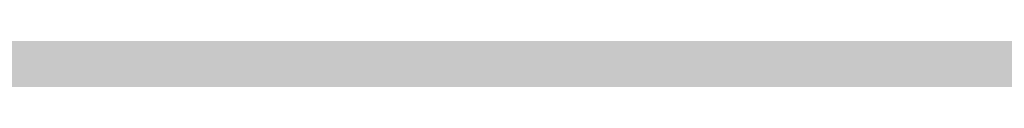
# Model space of a CAD drawing. Units: inches. Extents: x 2083 to 3317, y 1141 to 2115.
# Tile 152 of 256: x 3126.946713 to 3126.955939, y 1263.261646 to 1263.261932. Entities that reach past the tile are written whole.
import ezdxf

# ---------------------------------------------------------------- set-up
doc = ezdxf.new("R2010")
doc.units = ezdxf.units.IN
doc.layers.add('A-ANNO-DIMS', color=2, linetype='Continuous', lineweight=18)
doc.layers.add('A-WALL-PATT', color=251, linetype='Continuous', lineweight=13, true_color=0x636466)
doc.styles.get("Standard").update_dxf_attribs({"font": 'arial.ttf'})
doc.dimstyles.new('ISO-25', dxfattribs={"dimtxt": 12, "dimasz": 12, "dimexe": 1.25, "dimexo": 0.625, "dimtad": 1, "dimlunit": 3, "dimtxsty": 'Standard', "dimcen": 2.5, "dimadec": 0, "dimazin": 0, "dimtfac": 1, "dimtmove": 0, "dimatfit": 3, "dimfxl": 1, "dimarcsym": 0})

# ---------------------------------------------------------------- blocks, each defined once
blk = doc.blocks.new('*D26')
at = {"layer": 'A-ANNO-DIMS', "color": 0, "lineweight": -2, "transparency": 16777216}
for p, q in [((3088.985844, 1274.915092), (3088.985844, 1270.9519631)), ((3111.2400366, 1274.915092), (3111.2400366, 1270.9519631)), ((3076.985844, 1272.2019631), (2840.262447, 1272.2019631)), ((3111.2400366, 1272.2019631), (3088.985844, 1272.2019631)), ((3123.2400366, 1272.2019631), (3135.2400366, 1272.2019631))]:
    blk.add_line(p, q, dxfattribs=at)
at = {"layer": 'A-ANNO-DIMS', "color": 0, "transparency": 16777216}
for points in [[(3076.985844, 1274.2019631), (3076.985844, 1270.2019631), (3088.985844, 1272.2019631)], [(3123.2400366, 1274.2019631), (3123.2400366, 1270.2019631), (3111.2400366, 1272.2019631)]]:
    blk.add_solid(points, dxfattribs=at)
at = {"layer": 'Defpoints', "color": 0, "transparency": 16777216}
for p in [(3088.985844, 1275.540092), (3111.2400366, 1275.540092), (3088.985844, 1272.2019631)]:
    blk.add_point(p, dxfattribs=at)
at = {"layer": 'A-ANNO-DIMS', "color": 0, "transparency": 16777216, "insert": (2952.6241455, 1279.0316016), "char_height": 12, "attachment_point": 5}
blk.add_mtext('NIGHTSTAND 1\'-10 1/2" TYP.', dxfattribs=at)

msp = doc.modelspace()

# ---------------------------------------------------------------- hatches: boundary and pattern name
at = {"layer": 'A-WALL-PATT'}
h = msp.add_hatch(color=256, dxfattribs=at)
h.dxf.hatch_style = 1
h.paths.add_polyline_path([(3126.9597832, 2020.7613601), (2748.9597832, 2020.7613601), (2604.9597832, 2020.7613601), (2226.9597832, 2020.7613601), (2226.9597832, 1702.7613601), (2466.9597832, 1702.7613601), (2466.9597832, 1582.7613601), (2418.9597832, 1582.7613601), (2418.9597832, 1477.7613601), (2226.9597832, 1477.7613601), (2226.9597832, 1263.2613601), (2544.9597832, 1263.2613601), (2544.9597832, 1411.7613601), (2604.9597832, 1411.7613601), (2685.9597832, 1411.7613601), (2685.9597832, 1420.7613601), (2604.9597832, 1420.7613601), (2604.9597832, 1573.7613601), (2604.9597832, 1702.7613601), (2604.9597832, 2011.7613601), (2748.9597832, 2011.7613601), (2748.9597832, 1702.7613601), (2862.9597832, 1702.7613601), (2862.9597832, 1621.7613601), (2871.9597832, 1621.7613601), (2871.9597832, 1702.7613601), (2883.9597832, 1702.7613601), (2883.9597832, 1706.9394595, -0.026459), (2883.9597832, 1711.7613601), (2757.9597832, 1711.7613601), (2757.9597832, 1807.7613601), (2787.9597832, 1807.7613601), (2787.9597832, 1812.2613601), (2757.9597832, 1812.2613601), (2757.9597832, 2011.7613601), (2877.9597832, 2011.7613601), (2877.9597832, 1812.2613601), (2847.9597832, 1812.2613601), (2847.9597832, 1807.7613601), (2889.8357425, 1807.7613601), (2889.8357425, 1812.2613601), (2882.4597832, 1812.2613601), (2882.4597832, 2011.7613601), (3117.9597832, 2011.7613601), (3117.9597832, 1812.2613601), (2937.8357425, 1812.2613601), (2937.8357425, 1807.7613601), (2995.7097832, 1807.7613601), (2995.7097832, 1796.1176655), (3000.2097832, 1796.1176655), (3000.2097832, 1807.7613601), (3117.9597832, 1807.7613601), (3117.9597832, 1711.7613601), (3000.2097832, 1711.7613601), (3000.2097832, 1760.1176655), (2998.5727047, 1760.1176655, -0.020711), (2995.7097832, 1760.1176655), (2995.7097832, 1711.7613601), (2931.9597832, 1711.7613601), (2931.9597832, 1702.7613601), (3126.9597832, 1702.7613601)])
h.paths.add_polyline_path([(2471.4597832, 2011.7613601), (2471.4597832, 1810.0113601), (2462.7169357, 1810.0113601), (2462.7169357, 1805.5113601), (2505.9597832, 1805.5113601), (2505.9597832, 1810.0113601), (2475.9597832, 1810.0113601), (2475.9597832, 2011.7613601), (2595.9597832, 2011.7613601), (2595.9597832, 1810.0113601), (2565.9597832, 1810.0113601), (2565.9597832, 1805.5113601), (2595.9597832, 1805.5113601), (2595.9597832, 1711.7613601), (2235.9597832, 1711.7613601), (2235.9597832, 1805.5113601), (2353.7097832, 1805.5113601), (2353.7097832, 1796.0541624), (2358.2097832, 1796.0541624), (2358.2097832, 1805.5113601), (2414.7169357, 1805.5113601), (2414.7169357, 1810.0113601), (2235.9597832, 1810.0113601), (2235.9597832, 2011.7613601)], flags=16)
h.paths.add_polyline_path([(2270.2047343, 1994.6100082), (2270.2047343, 1970.6100082), (2246.2047343, 1970.6100082), (2246.2047343, 1994.6100082)], flags=0)
edge = h.paths.add_edge_path(flags=0)
edge.add_ellipse((2332.027391, 1899.7981761), major_axis=(-3.0429938, 3.0429938), ratio=0.16825245, start_angle=-161.3321656, end_angle=-156.3071136, ccw=False)
edge.add_ellipse((2333.0820373, 1898.7435297), major_axis=(-1.0546463, 1.0546463), ratio=0.453532097, start_angle=-123.371019, end_angle=-94.1591066)
edge = h.paths.add_edge_path(flags=0)
edge.add_ellipse((2332.027391, 1968.8762897), major_axis=(3.0429938, 3.0429938), ratio=0.16825245, start_angle=18.6678344, end_angle=23.6928864)
edge.add_spline(control_points=[(2332.9255964, 1970.6911045), (2332.2267681, 1970.3360997), (2330.8937087, 1969.6589054), (2328.4130803, 1970.9321376), (2327.2039345, 1967.7487119), (2324.7095965, 1969.9555886), (2322.5328223, 1967.012354), (2320.0128462, 1971.2958124), (2317.6803077, 1968.1578449), (2316.0405263, 1967.1020468), (2315.4269045, 1966.8096022)], knot_values=[0, 0, 0, 0, 2.267059, 4.324559, 6.685584, 8.878641, 11.121502, 14.300359, 17.755284, 19.732645, 19.732645, 19.732645, 19.732645], degree=3, periodic=0)
edge.add_ellipse((2332.027391, 1968.8762897), major_axis=(3.0429938, 3.0429938), ratio=0.16825245, start_angle=18.6678344, end_angle=23.6928864, ccw=False)
edge.add_ellipse((2333.0820373, 1969.930936), major_axis=(1.0546463, 1.0546463), ratio=0.453532097, start_angle=56.628981, end_angle=85.8408934, ccw=False)
edge = h.paths.add_edge_path(flags=0)
edge.add_spline(control_points=[(2296.4282874, 1967.9879081), (2293.6278045, 1965.3363137), (2287.7036238, 1959.727094), (2299.7438601, 1949.9956993), (2294.5325909, 1935.6685275), (2290.5732281, 1920.6035119), (2293.3941244, 1909.9736911), (2296.1854073, 1904.9665431)], knot_values=[0.099185, 0.099185, 0.099185, 0.099185, 0.345301, 0.619822, 0.982653, 1.386093, 1.810555, 1.810555, 1.810555, 1.810555], degree=3, periodic=0)
edge.add_spline(control_points=[(2296.1854073, 1904.9665431), (2297.3835817, 1902.6193002), (2298.0009694, 1901.9493116), (2298.5529698, 1901.4681549)], knot_values=[0.006246, 0.006246, 0.006246, 0.006246, 0.055476, 0.055476, 0.055476, 0.055476], degree=3, periodic=0)
edge.add_spline(control_points=[(2298.5529698, 1901.4681549), (2297.2586121, 1900.9232238), (2295.2252939, 1900.2321257), (2293.0602287, 1900.6142053), (2292.1014227, 1900.788415), (2292.0895776, 1900.790568)], knot_values=[0.312835, 0.312835, 0.312835, 0.312835, 0.40178, 0.474987, 0.475903, 0.475903, 0.475903, 0.475903], degree=3, periodic=0)
edge.add_arc((2292.7936464, 1904.6641088), 3.9370079, 215.4208969, 259.6981795, ccw=False)
edge.add_spline(control_points=[(2289.5853139, 1902.3823039), (2289.4766524, 1902.5350874), (2289.3684805, 1902.6880353), (2289.2608648, 1902.8411699)], knot_values=[0.102872, 0.102872, 0.102872, 0.102872, 0.116896, 0.116896, 0.116896, 0.116896], degree=3, periodic=0)
edge.add_spline(control_points=[(2289.2608648, 1902.8411699), (2288.6866042, 1902.5501922), (2287.6400477, 1902.0199025), (2285.8813368, 1901.8739536), (2283.8529717, 1901.5043521), (2281.7199871, 1899.7105375), (2278.4669913, 1899.492942), (2276.1571361, 1901.8832022), (2272.2589526, 1899.8040711), (2267.7776054, 1901.8431828), (2262.2438819, 1900.1840326), (2257.414927, 1901.7820606), (2254.318374, 1900.7261196), (2253.1782849, 1900.3373431)], knot_values=[0, 0, 0, 0, 1.907977, 3.477176, 5.261074, 7.972851, 11.680248, 13.717921, 16.939592, 22.789562, 27.502503, 33.595215, 37.145618, 37.145618, 37.145618, 37.145618], degree=3, periodic=0)
edge.add_line((2253.1782849, 1900.3373431), (2250.2442397, 1902.8411699))
edge.add_line((2250.2442397, 1902.8411699), (2250.2442397, 1965.8332959))
edge.add_line((2250.2442397, 1965.8332959), (2253.1782849, 1968.3371226))
edge.add_spline(control_points=[(2253.1782849, 1968.3371226), (2254.318374, 1967.9483462), (2257.414927, 1966.8924051), (2262.2438819, 1968.4904332), (2267.7776054, 1966.8312829), (2271.5267301, 1968.5372172), (2273.8759143, 1967.8282895), (2274.2067012, 1967.7276424)], knot_values=[0, 0, 0, 0, 0.09018, 0.244935, 0.364644, 0.513233, 0.537855, 0.537855, 0.537855, 0.537855], degree=3, periodic=0)
edge.add_arc((2274.3528869, 1963.7933495), 3.9370079, 72.0511336, 92.1279492, ccw=False)
edge.add_arc((2281.2969331, 1985.2300027), 18.5962982, 252.05113361, 288.56572166)
edge.add_arc((2292.3167172, 1956.0288805), 12.6460805, 71.02678788, 113.77821843, ccw=False)
edge = h.paths.add_edge_path(flags=0)
edge.add_spline(control_points=[(2274.8994147, 1951.8561946), (2275.066156, 1951.6165924), (2275.2326866, 1951.3765878), (2275.3979871, 1951.1358545)], knot_values=[1.409916, 1.409916, 1.409916, 1.409916, 1.43159, 1.43159, 1.43159, 1.43159], degree=3, periodic=0)
edge.add_spline(control_points=[(2275.3979871, 1951.1358545), (2275.7921055, 1950.5618854), (2276.1792311, 1949.9837745), (2276.5455462, 1949.3971029)], knot_values=[1.358238, 1.358238, 1.358238, 1.358238, 1.409916, 1.409916, 1.409916, 1.409916], degree=3, periodic=0)
edge.add_line((2276.5455462, 1949.3971029), (2277.437289, 1947.8621847))
edge.add_spline(control_points=[(2277.437289, 1947.8621847), (2276.3038341, 1945.6731147), (2274.6396979, 1942.4268817), (2274.631615, 1938.0938998), (2272.7991237, 1930.8515498), (2274.3564261, 1943.8970461), (2275.9476814, 1947.9233558), (2276.5455462, 1949.3971029)], knot_values=[0.005632, 0.005632, 0.005632, 0.005632, 0.186014, 0.266002, 0.357087, 0.59639, 0.739732, 0.739732, 0.739732, 0.739732], degree=3, periodic=0)
edge.add_spline(control_points=[(2276.5455462, 1949.3971029), (2276.1792311, 1949.9837745), (2275.7921055, 1950.5618854), (2275.3979871, 1951.1358545)], knot_values=[1.358238, 1.358238, 1.358238, 1.358238, 1.409916, 1.409916, 1.409916, 1.409916], degree=3, periodic=0)
edge.add_spline(control_points=[(2275.3979871, 1951.1358545), (2274.9425002, 1950.0804523), (2274.2077604, 1948.0252718), (2273.9346018, 1944.8514774), (2272.4685341, 1937.6274891), (2273.4662155, 1945.6964663), (2274.7006154, 1951.0594725), (2274.8994147, 1951.8561946)], knot_values=[0.104364, 0.104364, 0.104364, 0.104364, 0.189636, 0.269624, 0.36071, 0.600013, 0.644622, 0.644622, 0.644622, 0.644622], degree=3, periodic=0)
h.paths.add_polyline_path([(2269.1675139, 1963.1275729, -0.357527), (2268.170633, 1960.9763695, -0.092561), (2268.170633, 1939.4363249, -0.357527), (2269.1675139, 1937.2851215, -0.357527), (2267.0163105, 1938.2820024, -0.164785), (2254.6855813, 1938.2820024, -0.357527), (2252.5343779, 1937.2851215, -0.357527), (2253.5312587, 1939.4363249, -0.092561), (2253.5312587, 1960.9763695, -0.357527), (2252.5343779, 1963.1275729, -0.357527), (2254.6855813, 1962.130692, -0.164785), (2267.0163105, 1962.130692, -0.357527)], flags=0)
h.paths.add_polyline_path([(2248.8740679, 1967.8017998), (2248.8740679, 1957.0277095), (2249.4577833, 1957.0277095), (2249.4577833, 1911.6467562), (2248.8740679, 1911.6467562), (2248.8740679, 1900.8726659), (2246.5118632, 1900.8726659, 0.197327), (2244.1496584, 1902.4568734), (2244.1496584, 1966.2175923, 0.197327), (2246.5118632, 1967.8017998)], flags=0)
h.paths.add_polyline_path([(2269.1675139, 1931.3893442, -0.357527), (2268.170633, 1929.2381408, -0.092561), (2268.170633, 1907.6980962, -0.357527), (2269.1675139, 1905.5468928, -0.357527), (2267.0163105, 1906.5437737, -0.164785), (2254.6855813, 1906.5437737, -0.357527), (2252.5343779, 1905.5468928, -0.357527), (2253.5312587, 1907.6980962, -0.092561), (2253.5312587, 1929.2381408, -0.357527), (2252.5343779, 1931.3893442, -0.357527), (2254.6855813, 1930.3924634, -0.164785), (2267.0163105, 1930.3924634, -0.357527)], flags=0)
edge = h.paths.add_edge_path(flags=0)
edge.add_spline(control_points=[(2276.1968578, 1906.7237016), (2276.1681442, 1909.0289278), (2276.1140492, 1913.371852), (2270.5984171, 1924.9249783), (2273.9051746, 1919.0127787), (2275.9217115, 1916.2620626), (2275.4745699, 1912.4021495), (2277.2578735, 1910.3806206), (2276.6960436, 1908.2250358), (2276.6462176, 1906.8130226), (2276.6178249, 1906.0084068)], knot_values=[0, 0, 0, 0, 8.61026, 16.221274, 18.843057, 23.804898, 27.440828, 29.356102, 31.203478, 33.650687, 33.650687, 33.650687, 33.650687], degree=3, periodic=0)
edge.add_spline(control_points=[(2276.6178249, 1906.0084068), (2276.6233131, 1905.6241436), (2276.4977381, 1904.6286608), (2275.4417789, 1903.8547251), (2274.9373144, 1903.0804497), (2274.8590804, 1902.8411699)], knot_values=[0.156488, 0.156488, 0.156488, 0.156488, 0.184398, 0.231376, 0.250598, 0.250598, 0.250598, 0.250598], degree=3, periodic=0)
edge.add_line((2274.8590804, 1902.8411699), (2276.50598, 1902.8411699))
edge.add_spline(control_points=[(2276.50598, 1902.8411699), (2276.7883084, 1903.0849395), (2277.6650711, 1904.1251958), (2278.2495378, 1904.340738), (2277.6538719, 1908.5273866), (2278.15567, 1906.2278078), (2278.100464, 1905.2859484), (2278.8466748, 1904.0690054), (2277.8567853, 1903.4149482), (2277.8741909, 1902.9910497), (2277.9035616, 1902.8411699)], knot_values=[0.059574, 0.059574, 0.059574, 0.059574, 0.080753, 0.103741, 0.16972, 0.176036, 0.207137, 0.240474, 0.262341, 0.27366, 0.27366, 0.27366, 0.27366], degree=3, periodic=0)
edge.add_line((2277.9035616, 1902.8411699), (2280.0298255, 1902.8411699))
edge.add_spline(control_points=[(2280.0298255, 1902.8411699), (2279.8882214, 1903.088398), (2279.4992571, 1903.9815512), (2280.1522839, 1905.9393491), (2278.103615, 1909.6577572), (2279.7623946, 1907.185285), (2280.3279002, 1904.8748608), (2280.4851086, 1903.4895904), (2281.4632687, 1903.2494323), (2281.7583431, 1902.9364967), (2281.8340361, 1902.8411699)], knot_values=[0.013856, 0.013856, 0.013856, 0.013856, 0.034874, 0.088867, 0.107879, 0.126738, 0.158714, 0.193757, 0.217487, 0.226722, 0.226722, 0.226722, 0.226722], degree=3, periodic=0)
edge.add_spline(control_points=[(2281.8340361, 1902.8411699), (2281.7875348, 1902.8267029), (2281.6470224, 1902.7829881), (2281.3955272, 1902.85949), (2281.088077, 1902.9852418), (2280.7206826, 1903.060902), (2280.3334513, 1903.0257257), (2280.1247668, 1902.898879), (2280.0298255, 1902.8411699)], knot_values=[0, 0, 0, 0, 0.14413, 0.435517, 0.749276, 1.153046, 1.548371, 1.878348, 1.878348, 1.878348, 1.878348], degree=3, periodic=0)
edge.add_line((2280.0298255, 1902.8411699), (2277.9035616, 1902.8411699))
edge.add_spline(control_points=[(2277.9035616, 1902.8411699), (2277.892855, 1902.7958553), (2277.865396, 1902.6796374), (2277.6074793, 1902.6874828), (2277.2740503, 1902.8006999), (2276.8379209, 1902.6197745), (2276.5838074, 1902.7892611), (2276.50598, 1902.8411699)], knot_values=[0, 0, 0, 0, 0.127189, 0.326199, 0.628009, 1.24357, 1.515331, 1.515331, 1.515331, 1.515331], degree=3, periodic=0)
edge.add_line((2276.50598, 1902.8411699), (2274.8590804, 1902.8411699))
edge.add_spline(control_points=[(2274.8590804, 1902.8411699), (2274.8144367, 1902.8985868), (2274.7251297, 1903.013446), (2274.4934765, 1903.1189684), (2274.2442854, 1902.9605386), (2273.9371207, 1903.1849416), (2273.6140395, 1902.9831428), (2273.4083164, 1902.8830449), (2273.322254, 1902.8411699)], knot_values=[0, 0, 0, 0, 0.21843, 0.436957, 0.687977, 0.990379, 1.398396, 1.69185, 1.69185, 1.69185, 1.69185], degree=3, periodic=0)
edge.add_spline(control_points=[(2273.322254, 1902.8411699), (2273.6167403, 1903.445692), (2274.2739977, 1904.5382529), (2276.0272387, 1904.5737017), (2276.2069634, 1906.5836372), (2276.1968578, 1906.7237016)], knot_values=[0.012227, 0.012227, 0.012227, 0.012227, 0.059472, 0.106218, 0.134458, 0.134458, 0.134458, 0.134458], degree=3, periodic=0)
h.paths.add_polyline_path([(2270.7760538, 1897.7898284), (2270.7760538, 1873.7898284), (2246.7760538, 1873.7898284), (2246.7760538, 1897.7898284)], flags=0)
h.paths.add_polyline_path([(2353.7097832, 1760.0050593), (2353.7097832, 1760.0541624), (2358.2097832, 1760.0541624, -0.033729)], flags=0)
h.paths.add_polyline_path([(2321.8191188, 1737.5291862), (2341.9953271, 1737.5291862, -0.414214), (2343.2032727, 1736.3212406), (2343.2032727, 1721.0205964, -0.414214), (2341.9953271, 1719.8126508), (2321.8191188, 1719.8126508, -0.414214), (2320.6111732, 1721.0205964), (2320.6111732, 1736.3212406, -0.414214)], flags=0)
h.paths.add_polyline_path([(2324.2350099, 1736.3212406), (2339.5794359, 1736.3212406, -0.414214), (2341.9953271, 1733.9053494), (2341.9953271, 1725.4497302, -0.414214), (2339.5794359, 1723.033839), (2333.6805885, 1723.033839), (2333.8453172, 1722.0454666, -0.870646), (2335.4253988, 1721.8258934, -0.767327), (2333.922694, 1721.4232449), (2331.2910241, 1721.4232449, -0.767327), (2329.7883193, 1721.8258934, -0.870646), (2331.3684009, 1722.0454666), (2331.5331296, 1723.033839), (2324.2350099, 1723.033839, -0.414214), (2321.8191188, 1725.4497302), (2321.8191188, 1733.9053494, -0.414214)], flags=0)
h.paths.add_polyline_path([(2570.4837892, 1928.6154443), (2589.6837892, 1928.6154443), (2590.1688286, 1928.6154443), (2590.1688286, 1904.9933971), (2570.4837892, 1904.9933971)], flags=0)
h.paths.add_polyline_path([(2574.4473242, 1927.2638215, -1), (2572.8288357, 1927.2638215, -1)], flags=0)
h.paths.add_polyline_path([(2573.0898665, 1926.9408768), (2573.925032, 1927.7760423), (2574.1477428, 1927.5533315), (2573.3125773, 1926.718166)], flags=0)
h.paths.add_polyline_path([(2578.7790648, 1919.7296175, -1), (2571.5916632, 1919.7296175, -1)], flags=0)
h.paths.add_polyline_path([(2578.385364, 1919.7296175, -1), (2571.985364, 1919.7296175, -1)], flags=0)
h.paths.add_polyline_path([(2331.5957638, 1729.4762156, -1), (2333.6179542, 1729.4762156, -1)], flags=0)
h.paths.add_polyline_path([(2578.0342282, 1927.2638215, -1), (2576.4157396, 1927.2638215, -1)], flags=0)
h.paths.add_polyline_path([(2576.6888513, 1927.5310886), (2576.9115621, 1927.7537993), (2577.7467276, 1926.9186339), (2577.5240168, 1926.6959231)], flags=0)
h.paths.add_polyline_path([(2578.1390648, 1909.8595388, -1), (2572.2316632, 1909.8595388, -1)], flags=0)
h.paths.add_polyline_path([(2577.745364, 1909.8595388, -1), (2572.625364, 1909.8595388, -1)], flags=0)
h.paths.add_polyline_path([(2583.7977179, 1927.2638215, -1), (2582.1792294, 1927.2638215, -1)], flags=0)
h.paths.add_polyline_path([(2582.7186487, 1927.7537993), (2583.5538142, 1926.9186339), (2583.3311034, 1926.6959231), (2582.4959379, 1927.5310886)], flags=0)
h.paths.add_polyline_path([(2582.4959379, 1927.5310886), (2582.7186487, 1927.7537993), (2583.5538142, 1926.9186339), (2583.3311034, 1926.6959231)], flags=0)
h.paths.add_polyline_path([(2587.7390648, 1920.5296175, -1), (2581.8316632, 1920.5296175, -1)], flags=0)
h.paths.add_polyline_path([(2587.345364, 1920.5296175, -1), (2582.225364, 1920.5296175, -1)], flags=0)
h.paths.add_polyline_path([(2587.3846219, 1927.2638215, -1), (2585.7661333, 1927.2638215, -1)], flags=0)
h.paths.add_polyline_path([(2586.0819925, 1926.9802469), (2586.917158, 1927.8154124), (2587.1398688, 1927.5927016), (2586.3047033, 1926.7575361)], flags=0)
h.paths.add_polyline_path([(2588.3790648, 1910.6595388, -1), (2581.1916632, 1910.6595388, -1)], flags=0)
h.paths.add_polyline_path([(2587.985364, 1910.6595388, -1), (2581.585364, 1910.6595388, -1)], flags=0)
h.paths.add_polyline_path([(2417.1677288, 1729.4778955), (2437.3439372, 1729.4778955, -0.414214), (2438.5518828, 1728.2699499), (2438.5518828, 1712.9693057, -0.414214), (2437.3439372, 1711.7613601), (2417.1677288, 1711.7613601, -0.414214), (2415.9597832, 1712.9693057), (2415.9597832, 1728.2699499, -0.414214)], flags=0)
h.paths.add_polyline_path([(2419.58362, 1728.2699499), (2434.928046, 1728.2699499, -0.414214), (2437.3439372, 1725.8540587), (2437.3439372, 1717.3984395, -0.414214), (2434.928046, 1714.9825483), (2429.0291985, 1714.9825483), (2429.1939273, 1713.9941758, -0.870646), (2430.7740089, 1713.7746027, -0.767327), (2429.2713041, 1713.3719542), (2426.6396342, 1713.3719542, -0.767327), (2425.1369294, 1713.7746027, -0.870646), (2426.717011, 1713.9941758), (2426.8817397, 1714.9825483), (2419.58362, 1714.9825483, -0.414214), (2417.1677288, 1717.3984395), (2417.1677288, 1725.8540587, -0.414214)], flags=0)
h.paths.add_polyline_path([(2419.58362, 1728.2699499), (2434.928046, 1728.2699499, -0.414214), (2437.3439372, 1725.8540587), (2437.3439372, 1717.3984395, -0.414214), (2434.928046, 1714.9825483), (2429.0291985, 1714.9825483), (2428.3581177, 1719.0090337), (2427.5528206, 1719.0090337), (2426.8817397, 1714.9825483), (2419.58362, 1714.9825483, -0.414214), (2417.1677288, 1717.3984395), (2417.1677288, 1725.8540587, -0.414214)], flags=0)
h.paths.add_polyline_path([(2426.9443739, 1721.4249248, -1), (2428.9665643, 1721.4249248, -1)], flags=0)
h.paths.add_polyline_path([(2475.9597832, 1702.7613601), (2595.9597832, 1702.7613601), (2595.9597832, 1582.7613601), (2475.9597832, 1582.7613601)], flags=16)
h.paths.add_polyline_path([(2427.9597832, 1573.7613601), (2595.9597832, 1573.7613601), (2595.9597832, 1468.7613601), (2595.9597832, 1420.7613601), (2384.4597832, 1420.7613601), (2384.4597832, 1468.7613601), (2427.9597832, 1468.7613601)], flags=16)
h.paths.add_polyline_path([(2379.9597832, 1468.7613601), (2379.9597832, 1420.7613601), (2235.9597832, 1420.7613601), (2235.9597832, 1468.7613601)], flags=16)
h.paths.add_polyline_path([(2317.8159962, 1466.695767), (2337.9922045, 1466.695767, -0.414214), (2339.2001501, 1465.4878214), (2339.2001501, 1450.1871771, -0.414214), (2337.9922045, 1448.9792315), (2317.8159962, 1448.9792315, -0.414214), (2316.6080506, 1450.1871771), (2316.6080506, 1465.4878214, -0.414214)], flags=0)
h.paths.add_polyline_path([(2320.2318874, 1465.4878214), (2335.5763133, 1465.4878214, -0.414214), (2337.9922045, 1463.0719302), (2337.9922045, 1454.616311, -0.414214), (2335.5763133, 1452.2004198), (2329.6774659, 1452.2004198), (2329.8421946, 1451.2120473, -0.870646), (2331.4222762, 1450.9924742, -0.767327), (2329.9195714, 1450.5898257), (2327.2879015, 1450.5898257, -0.767327), (2325.7851967, 1450.9924742, -0.870646), (2327.3652783, 1451.2120473), (2327.530007, 1452.2004198), (2320.2318874, 1452.2004198, -0.414214), (2317.8159962, 1454.616311), (2317.8159962, 1463.0719302, -0.414214)], flags=0)
h.paths.add_polyline_path([(2320.2318874, 1465.4878214), (2335.5763133, 1465.4878214, -0.414214), (2337.9922045, 1463.0719302), (2337.9922045, 1454.616311, -0.414214), (2335.5763133, 1452.2004198), (2329.6774659, 1452.2004198), (2329.006385, 1456.2269051), (2328.2010879, 1456.2269051), (2327.530007, 1452.2004198), (2320.2318874, 1452.2004198, -0.414214), (2317.8159962, 1454.616311), (2317.8159962, 1463.0719302, -0.414214)], flags=0)
h.paths.add_polyline_path([(2327.5926413, 1458.6427963, -1), (2329.6148317, 1458.6427963, -1)], flags=0)
h.paths.add_polyline_path([(2244.4117436, 1433.3404531), (2241.9209449, 1433.3404531, -0.414214), (2240.0178562, 1435.2435418), (2240.0178562, 1440.9528078, -0.414211), (2241.920925, 1442.8558965), (2244.4117436, 1442.8558965, -1.976472)], flags=0)
h.paths.add_polyline_path([(2245.3568884, 1434.3975358, -0.414214), (2245.3568884, 1441.7988138, -2.144098)], flags=0)
h.paths.add_polyline_path([(2535.9597832, 1416.2613601), (2535.9597832, 1272.2613601), (2235.9597832, 1272.2613601), (2235.9597832, 1416.2613601)], flags=16)
h.paths.add_polyline_path([(2260.1195614, 1384.2928413), (2260.1195614, 1362.0386487), (2237.8653688, 1362.0386487), (2237.8653688, 1384.2928413)], flags=0)
edge = h.paths.add_edge_path(flags=0)
edge.add_line((2318.2518466, 1362.0932983), (2318.1457968, 1362.0009726))
edge.add_ellipse((2317.4451158, 1360.4310442), major_axis=(2.8216404, 2.8216404), ratio=0.16825245, start_angle=18.6678344, end_angle=20.9481273, ccw=False)
edge.add_ellipse((2318.4230451, 1361.4089735), major_axis=(0.9779293, 0.9779293), ratio=0.453532097, start_angle=56.628981, end_angle=70.2262012, ccw=False)
edge = h.paths.add_edge_path(flags=0)
edge.add_line((2319.1073699, 1295.5710784), (2319.0150442, 1295.6771282))
edge.add_ellipse((2317.4451158, 1296.3778091), major_axis=(-2.8216404, 2.8216404), ratio=0.16825245, start_angle=-161.3321656, end_angle=-159.0518727, ccw=False)
edge.add_ellipse((2318.4230451, 1295.3998798), major_axis=(-0.9779293, 0.9779293), ratio=0.453532097, start_angle=-123.371019, end_angle=-109.7737988)
edge = h.paths.add_edge_path(flags=0)
edge.add_spline(control_points=[(2284.2103489, 1301.1702189), (2284.5806878, 1300.444719), (2284.8911891, 1299.8920243), (2285.159553, 1299.4610182)], knot_values=[0.039066, 0.039066, 0.039066, 0.039066, 0.055476, 0.055476, 0.055476, 0.055476], degree=3, periodic=0)
edge.add_line((2285.159553, 1299.4610182), (2284.2103489, 1301.1702189))
edge = h.paths.add_edge_path(flags=0)
edge.add_line((2280.4124579, 1297.2980125), (2283.3699905, 1297.0361216))
edge.add_line((2283.3699905, 1297.0361216), (2286.4056902, 1297.9263104))
edge.add_spline(control_points=[(2286.4056902, 1297.9263104), (2285.305487, 1297.4631193), (2284.3447774, 1297.1291508), (2283.3699905, 1297.0361216)], knot_values=[0.394369, 0.394369, 0.394369, 0.394369, 0.475903, 0.475903, 0.475903, 0.475903], degree=3, periodic=0)
edge.add_spline(control_points=[(2283.3699905, 1297.0361216), (2283.2813895, 1297.027666), (2282.316289, 1296.9573356), (2281.3125019, 1297.1344787), (2280.4234414, 1297.2960161), (2280.4124579, 1297.2980125)], knot_values=[0.312835, 0.312835, 0.312835, 0.312835, 0.320246, 0.393453, 0.394369, 0.394369, 0.394369, 0.394369], degree=3, periodic=0)
edge = h.paths.add_edge_path(flags=0)
edge.add_line((2284.4355615, 1359.6072854), (2280.4462909, 1355.328047))
edge.add_line((2280.4462909, 1355.328047), (2279.5799868, 1351.0177544))
edge.add_line((2279.5799868, 1351.0177544), (2282.4129737, 1346.5804327))
edge.add_spline(control_points=[(2282.4129737, 1346.5804327), (2283.1533308, 1345.5892358), (2284.2528957, 1344.0288973), (2284.801037, 1342.3871671), (2284.9351625, 1341.8055443)], knot_values=[1.240098, 1.240098, 1.240098, 1.240098, 1.332892, 1.382712, 1.382712, 1.382712, 1.382712], degree=3, periodic=0)
edge.add_spline(control_points=[(2284.9351625, 1341.8055443), (2285.3191079, 1340.1406002), (2285.2330291, 1338.4092041), (2284.9099384, 1336.6541222)], knot_values=[1.097484, 1.097484, 1.097484, 1.097484, 1.240098, 1.240098, 1.240098, 1.240098], degree=3, periodic=0)
edge.add_spline(control_points=[(2284.9099384, 1336.6541222), (2284.5868478, 1334.8990403), (2284.0267453, 1333.1202725), (2283.4626437, 1331.3605849)], knot_values=[0.95487, 0.95487, 0.95487, 0.95487, 1.097484, 1.097484, 1.097484, 1.097484], degree=3, periodic=0)
edge.add_line((2283.4626437, 1331.3605849), (2281.8903759, 1326.153357))
edge.add_line((2281.8903759, 1326.153357), (2280.7562592, 1321.0560888))
edge.add_line((2280.7562592, 1321.0560888), (2280.2992048, 1316.0019772))
edge.add_line((2280.2992048, 1316.0019772), (2280.7159327, 1310.9500678))
edge.add_line((2280.7159327, 1310.9500678), (2282.0280939, 1305.9721367))
edge.add_line((2282.0280939, 1305.9721367), (2284.2103489, 1301.1702189))
edge.add_spline(control_points=[(2284.2103489, 1301.1702189), (2283.3407305, 1302.7301854), (2282.6119044, 1304.3364933), (2282.0280939, 1305.9721367)], knot_values=[0.099185, 0.099185, 0.099185, 0.099185, 0.241799, 0.241799, 0.241799, 0.241799], degree=3, periodic=0)
edge.add_spline(control_points=[(2282.0280939, 1305.9721367), (2281.4442835, 1307.6077801), (2281.0054886, 1309.2727591), (2280.7159327, 1310.9500678)], knot_values=[0.241799, 0.241799, 0.241799, 0.241799, 0.384413, 0.384413, 0.384413, 0.384413], degree=3, periodic=0)
edge.add_spline(control_points=[(2280.7159327, 1310.9500678), (2280.4332411, 1312.5876134), (2280.2893863, 1314.2769594), (2280.2988938, 1315.9620324), (2280.2992048, 1316.0019772)], knot_values=[0.384413, 0.384413, 0.384413, 0.384413, 0.523647, 0.527028, 0.527028, 0.527028, 0.527028], degree=3, periodic=0)
edge.add_spline(control_points=[(2280.2992048, 1316.0019772), (2280.3123257, 1317.6869552), (2280.4778706, 1319.3679256), (2280.7562592, 1321.0560888)], knot_values=[0.527028, 0.527028, 0.527028, 0.527028, 0.669642, 0.669642, 0.669642, 0.669642], degree=3, periodic=0)
edge.add_spline(control_points=[(2280.7562592, 1321.0560888), (2281.0346478, 1322.7442519), (2281.4258801, 1324.4396079), (2281.8903759, 1326.153357)], knot_values=[0.669642, 0.669642, 0.669642, 0.669642, 0.812256, 0.812256, 0.812256, 0.812256], degree=3, periodic=0)
edge.add_spline(control_points=[(2281.8903759, 1326.153357), (2282.2643834, 1327.5332507), (2282.7878702, 1329.2618097), (2283.352751, 1331.0177803), (2283.4626437, 1331.3605849)], knot_values=[0.812256, 0.812256, 0.812256, 0.812256, 0.927087, 0.95487, 0.95487, 0.95487, 0.95487], degree=3, periodic=0)
edge.add_line((2283.4626437, 1331.3605849), (2284.9099384, 1336.6541222))
edge.add_line((2284.9099384, 1336.6541222), (2284.9351625, 1341.8055443))
edge.add_line((2284.9351625, 1341.8055443), (2282.4129737, 1346.5804327))
edge.add_spline(control_points=[(2282.4129737, 1346.5804327), (2281.2751273, 1348.1037918), (2280.0784467, 1349.5703178), (2279.5799868, 1351.0177544)], knot_values=[1.382712, 1.382712, 1.382712, 1.382712, 1.525326, 1.525326, 1.525326, 1.525326], degree=3, periodic=0)
edge.add_spline(control_points=[(2279.5799868, 1351.0177544), (2279.4432818, 1351.4147209), (2279.1363124, 1352.856922), (2279.7351897, 1354.2903851), (2280.4462909, 1355.328047)], knot_values=[1.525326, 1.525326, 1.525326, 1.525326, 1.564439, 1.667941, 1.667941, 1.667941, 1.667941], degree=3, periodic=0)
edge.add_spline(control_points=[(2280.4462909, 1355.328047), (2281.4261132, 1356.7578354), (2282.9308373, 1358.1825604), (2284.4355615, 1359.6072854)], knot_values=[1.667941, 1.667941, 1.667941, 1.667941, 1.810555, 1.810555, 1.810555, 1.810555], degree=3, periodic=0)
edge.add_arc((2280.6230749, 1348.518181), 11.7261796, 71.02678788, 113.77821843)
edge.add_arc((2270.4048917, 1375.5951559), 17.2435667, 252.05113361, 288.56572166, ccw=False)
edge.add_arc((2263.9659692, 1355.7178471), 3.6506221, 72.0511336, 92.1279492)
edge.add_arc((2263.9659692, 1355.7178471), 3.6506221, 92.1279492, 177.98513)
edge.add_spline(control_points=[(2260.3176041, 1355.8461989), (2260.2604169, 1354.2206683), (2260.551278, 1350.1865469), (2262.9993445, 1346.7662507), (2264.4727415, 1344.6490245)], knot_values=[1.43159, 1.43159, 1.43159, 1.43159, 1.564144, 1.770695, 1.770695, 1.770695, 1.770695], degree=3, periodic=0)
edge.add_line((2264.4727415, 1344.6490245), (2264.9355904, 1343.9825301))
edge.add_spline(control_points=[(2263.8010444, 1340.2481052), (2263.8432379, 1340.5140884), (2264.0672444, 1341.7564652), (2264.5126928, 1343.0024532), (2264.9350468, 1343.9810834)], knot_values=[0.53657, 0.53657, 0.53657, 0.53657, 0.559349, 0.644622, 0.644622, 0.644622, 0.644622], degree=3, periodic=0)
edge.add_spline(control_points=[(2264.9350468, 1343.9810834), (2265.1177715, 1343.7149747), (2265.2988751, 1343.4479058), (2265.4767562, 1343.1793646)], knot_values=[1.384077, 1.384077, 1.384077, 1.384077, 1.409916, 1.409916, 1.409916, 1.409916], degree=3, periodic=0)
edge.add_spline(control_points=[(2265.4767562, 1343.1793646), (2265.6546373, 1342.9108234), (2265.8292958, 1342.64081), (2265.9991301, 1342.368812)], knot_values=[1.358238, 1.358238, 1.358238, 1.358238, 1.384077, 1.384077, 1.384077, 1.384077], degree=3, periodic=0)
edge.add_line((2265.9991301, 1342.368812), (2266.8260057, 1340.9455468))
edge.add_spline(control_points=[(2266.8260057, 1340.9455468), (2268.894401, 1337.0896912), (2271.3981727, 1325.8430009), (2270.5161644, 1310.5685568), (2275.9193759, 1301.860609), (2277.7895113, 1299.1994495)], knot_values=[0.116896, 0.116896, 0.116896, 0.116896, 0.472987, 1.050969, 1.313793, 1.313793, 1.313793, 1.313793], degree=3, periodic=0)
edge.add_spline(control_points=[(2277.7895113, 1299.1994495), (2277.8394051, 1299.1284519), (2277.8894277, 1299.0574975), (2277.9395717, 1298.9865839)], knot_values=[0.109884, 0.109884, 0.109884, 0.109884, 0.116896, 0.116896, 0.116896, 0.116896], degree=3, periodic=0)
edge.add_line((2277.9395717, 1298.9865839), (2277.7888489, 1299.1991139))
edge.add_spline(control_points=[(2277.7888489, 1299.1991139), (2277.2565819, 1298.9294144), (2276.2863504, 1298.4379024), (2275.0393517, 1298.3344186), (2274.3833299, 1298.2388951), (2274.2152543, 1298.209338)], knot_values=[33.12187, 33.12187, 33.12187, 33.12187, 35.029056, 36.598255, 37.144827, 37.144827, 37.144827, 37.144827], degree=3, periodic=0)
edge.add_line((2274.2152543, 1298.209338), (2273.073147, 1297.8929607))
edge.add_spline(control_points=[(2273.073147, 1297.8929607), (2272.3229363, 1297.579784), (2271.0391507, 1296.5105078), (2269.2483948, 1296.2260622), (2268.4231004, 1296.3746543)], knot_values=[26.532584, 26.532584, 26.532584, 26.532584, 29.198919, 31.839101, 31.839101, 31.839101, 31.839101], degree=3, periodic=0)
edge.add_line((2268.4231004, 1296.3746543), (2263.8785014, 1297.4575338))
edge.add_spline(control_points=[(2263.8785014, 1297.4575338), (2263.5560769, 1297.3594345), (2261.8603064, 1296.8386943), (2260.2387805, 1297.2824073), (2258.9334543, 1297.5164611)], knot_values=[15.919551, 15.919551, 15.919551, 15.919551, 16.939592, 21.226067, 21.226067, 21.226067, 21.226067], degree=3, periodic=0)
edge.add_line((2258.9334543, 1297.5164611), (2254.0552332, 1297.3290098))
edge.add_spline(control_points=[(2254.0552332, 1297.3290098), (2253.7555255, 1297.295815), (2252.1136834, 1297.1651738), (2250.4618687, 1297.5442209), (2249.1296862, 1297.6678818)], knot_values=[5.306517, 5.306517, 5.306517, 5.306517, 6.276435, 10.613034, 10.613034, 10.613034, 10.613034], degree=3, periodic=0)
edge.add_line((2249.1296862, 1297.6678818), (2244.3316495, 1296.8777561))
edge.add_line((2244.3316495, 1296.8777561), (2241.6110326, 1299.1994495))
edge.add_line((2241.6110326, 1299.1994495), (2241.6110326, 1357.6094038))
edge.add_line((2241.6110326, 1357.6094038), (2244.3316495, 1359.9310973))
edge.add_line((2244.3316495, 1359.9310973), (2252.7288228, 1359.5426917))
edge.add_spline(control_points=[(2252.7288228, 1359.5426917), (2252.8709387, 1359.5464396), (2253.3057402, 1359.5481716), (2253.7398447, 1359.5142744), (2254.0317419, 1359.4824261)], knot_values=[0.233291, 0.233291, 0.233291, 0.233291, 0.244935, 0.268927, 0.268927, 0.268927, 0.268927], degree=3, periodic=0)
edge.add_line((2254.0317419, 1359.4824261), (2259.5871899, 1359.4163899))
edge.add_spline(control_points=[(2259.5871899, 1359.4163899), (2260.6770676, 1359.6285026), (2262.0731971, 1359.8970025), (2263.5236925, 1359.4592776), (2263.8304173, 1359.3659518)], knot_values=[0.422516, 0.422516, 0.422516, 0.422516, 0.513233, 0.537855, 0.537855, 0.537855, 0.537855], degree=3, periodic=0)
edge.add_arc((2263.9659692, 1355.7178471), 3.6506221, 72.0511336, 92.1279492, ccw=False)
edge.add_arc((2270.4048917, 1375.5951559), 17.2435667, 252.05113361, 288.56572166)
edge.add_arc((2280.6230749, 1348.518181), 11.7261796, 71.02678788, 113.77821843, ccw=False)
h.paths.add_polyline_path([(2240.3405298, 1359.4347149), (2240.3405298, 1349.4443532), (2240.8817846, 1349.4443532), (2240.8817846, 1307.3645001), (2240.3405298, 1307.3645001), (2240.3405298, 1297.3741385), (2238.1501565, 1297.3741385, 0.197327), (2235.9597832, 1298.8431076), (2235.9597832, 1357.9657458, 0.197327), (2238.1501565, 1359.4347149)], flags=0)
h.paths.add_polyline_path([(2259.1577904, 1355.1005005, -0.357527), (2258.2334246, 1353.1057799, -0.092561), (2258.2334246, 1333.1326007, -0.357527), (2259.1577904, 1331.1378801, -0.357527), (2257.1630698, 1332.0622458, -0.164785), (2245.7293022, 1332.0622458, -0.357527), (2243.7345816, 1331.1378801, -0.357527), (2244.6589474, 1333.1326007, -0.092561), (2244.6589474, 1353.1057799, -0.357527), (2243.7345816, 1355.1005005, -0.357527), (2245.7293022, 1354.1761347, -0.164785), (2257.1630698, 1354.1761347, -0.357527)], flags=0)
edge = h.paths.add_edge_path(flags=0)
edge.add_line((2265.9991301, 1342.368812), (2266.8260057, 1340.9455468))
edge.add_line((2266.8260057, 1340.9455468), (2265.3075567, 1337.8140664))
edge.add_line((2265.3075567, 1337.8140664), (2264.358232, 1334.6529388))
edge.add_line((2264.358232, 1334.6529388), (2264.2620123, 1333.7997046))
edge.add_spline(control_points=[(2264.2620123, 1333.7997046), (2264.2083565, 1333.187055), (2264.1620602, 1332.3655252), (2264.0071444, 1331.4139326), (2263.9690487, 1331.2018338)], knot_values=[0.464444, 0.464444, 0.464444, 0.464444, 0.516691, 0.531608, 0.531608, 0.531608, 0.531608], degree=3, periodic=0)
edge.add_spline(control_points=[(2263.9690487, 1331.2018338), (2263.7745349, 1330.1188727), (2263.4243703, 1328.7908386), (2263.2574202, 1328.5306516), (2263.2340282, 1328.5146115)], knot_values=[0.372682, 0.372682, 0.372682, 0.372682, 0.44885, 0.464444, 0.464444, 0.464444, 0.464444], degree=3, periodic=0)
edge.add_spline(control_points=[(2263.2340282, 1328.5146115), (2263.096382, 1328.4202271), (2263.1311696, 1329.3014765), (2263.2749528, 1330.6157493)], knot_values=[0.280919, 0.280919, 0.280919, 0.280919, 0.372682, 0.372682, 0.372682, 0.372682], degree=3, periodic=0)
edge.add_spline(control_points=[(2263.2749528, 1330.6157493), (2263.4187361, 1331.930022), (2263.6715151, 1333.677318), (2263.9698519, 1335.3150268)], knot_values=[0.189157, 0.189157, 0.189157, 0.189157, 0.280919, 0.280919, 0.280919, 0.280919], degree=3, periodic=0)
edge.add_spline(control_points=[(2263.9698519, 1335.3150268), (2264.1004958, 1336.0321917), (2264.4187827, 1337.6219113), (2264.7548476, 1338.8644304), (2264.9474193, 1339.4911244)], knot_values=[0.097394, 0.097394, 0.097394, 0.097394, 0.137578, 0.189157, 0.189157, 0.189157, 0.189157], degree=3, periodic=0)
edge.add_spline(control_points=[(2264.9474193, 1339.4911244), (2265.2900171, 1340.6060546), (2265.6442376, 1341.4939958), (2265.9991301, 1342.368812)], knot_values=[0.005632, 0.005632, 0.005632, 0.005632, 0.097394, 0.097394, 0.097394, 0.097394], degree=3, periodic=0)
h.paths.add_polyline_path([(2259.1577904, 1325.6709733, -0.357527), (2258.2334246, 1323.6762527, -0.092561), (2258.2334246, 1303.7030735, -0.357527), (2259.1577904, 1301.7083529, -0.357527), (2257.1630698, 1302.6327186, -0.164785), (2245.7293022, 1302.6327186, -0.357527), (2243.7345816, 1301.7083529, -0.357527), (2244.6589474, 1303.7030735, -0.092561), (2244.6589474, 1323.6762527, -0.357527), (2243.7345816, 1325.6709733, -0.357527), (2245.7293022, 1324.7466075, -0.164785), (2257.1630698, 1324.7466075, -0.357527)], flags=0)
edge = h.paths.add_edge_path(flags=0)
edge.add_spline(control_points=[(2261.7089377, 1317.3114208), (2261.6794818, 1317.4175798), (2261.7618581, 1317.3885347), (2262.4907358, 1316.0898725), (2262.962185, 1315.3008975)], knot_values=[14.955861, 14.955861, 14.955861, 14.955861, 16.221274, 18.694826, 18.694826, 18.694826, 18.694826], degree=3, periodic=0)
edge.add_spline(control_points=[(2262.962185, 1315.3008975), (2262.9904374, 1315.2536169), (2263.7020958, 1314.0673762), (2264.3489834, 1313.1271533), (2264.7300545, 1312.1641544)], knot_values=[18.694826, 18.694826, 18.694826, 18.694826, 18.843057, 22.433791, 22.433791, 22.433791, 22.433791], degree=3, periodic=0)
edge.add_spline(control_points=[(2264.7300545, 1312.1641544), (2264.8755649, 1311.7964373), (2265.1768733, 1310.7698073), (2265.1430689, 1309.5592623), (2265.2477363, 1308.8241926)], knot_values=[22.433791, 22.433791, 22.433791, 22.433791, 23.804898, 26.172756, 26.172756, 26.172756, 26.172756], degree=3, periodic=0)
edge.add_line((2265.2477363, 1308.8241926), (2265.8507741, 1307.1718879))
edge.add_spline(control_points=[(2265.8507741, 1307.1718879), (2266.0650246, 1306.8216779), (2266.3843872, 1306.3322461), (2266.4244001, 1305.7805489), (2266.4203688, 1305.6112163)], knot_values=[28.062562, 28.062562, 28.062562, 28.062562, 29.356102, 29.911721, 29.911721, 29.911721, 29.911721], degree=3, periodic=0)
edge.add_spline(control_points=[(2266.4203688, 1305.6112163), (2266.4161162, 1305.4325896), (2266.393999, 1305.2499979), (2266.3647773, 1305.0658571)], knot_values=[29.911721, 29.911721, 29.911721, 29.911721, 30.497837, 30.497837, 30.497837, 30.497837], degree=3, periodic=0)
edge.add_line((2266.3647773, 1305.0658571), (2266.0661511, 1302.1362954))
edge.add_spline(control_points=[(2266.0661511, 1302.1362954), (2266.0712401, 1301.7799843), (2265.9980761, 1301.1999847), (2265.6632664, 1300.7589613), (2265.5089084, 1300.5858824)], knot_values=[0.156488, 0.156488, 0.156488, 0.156488, 0.184398, 0.203543, 0.203543, 0.203543, 0.203543], degree=3, periodic=0)
edge.add_line((2265.5089084, 1300.5858824), (2264.4353411, 1299.1994495))
edge.add_line((2264.4353411, 1299.1994495), (2265.962442, 1299.1994495))
edge.add_line((2265.962442, 1299.1994495), (2267.3359898, 1301.1752758))
edge.add_line((2267.3359898, 1301.1752758), (2267.3116668, 1301.9862366))
edge.add_spline(control_points=[(2267.3116668, 1301.9862366), (2267.261111, 1302.8623959), (2267.1602121, 1303.7371316), (2267.2714865, 1303.3258962)], knot_values=[0.126229, 0.126229, 0.126229, 0.126229, 0.166617, 0.166617, 0.166617, 0.166617], degree=3, periodic=0)
edge.add_spline(control_points=[(2267.2714865, 1303.3258962), (2267.2800347, 1303.2943047), (2267.3097851, 1303.1753659), (2267.3734504, 1302.8836084), (2267.4061233, 1302.6828291), (2267.4179259, 1302.6010251)], knot_values=[0.166617, 0.166617, 0.166617, 0.166617, 0.16972, 0.176036, 0.180765, 0.180765, 0.180765, 0.180765], degree=3, periodic=0)
edge.add_spline(control_points=[(2267.7438914, 1300.9875045), (2267.6875832, 1301.1509426), (2267.4805198, 1301.6566644), (2267.4837514, 1302.1447877), (2267.4179259, 1302.6010251)], knot_values=[0.180765, 0.180765, 0.180765, 0.180765, 0.193767, 0.220139, 0.220139, 0.220139, 0.220139], degree=3, periodic=0)
edge.add_line((2267.4179259, 1302.6010251), (2267.7438914, 1300.9875045))
edge.add_spline(control_points=[(2267.7438914, 1300.9875045), (2267.8319608, 1300.7318778), (2267.9320205, 1300.3099042), (2267.5548409, 1299.9745185), (2267.429366, 1299.8292073)], knot_values=[0.220139, 0.220139, 0.220139, 0.220139, 0.240474, 0.25489, 0.25489, 0.25489, 0.25489], degree=3, periodic=0)
edge.add_line((2267.429366, 1299.8292073), (2267.2583608, 1299.1994495))
edge.add_line((2267.2583608, 1299.1994495), (2269.229956, 1299.1994495))
edge.add_spline(control_points=[(2269.229956, 1299.1994495), (2269.0986525, 1299.4286938), (2268.842774, 1300.0162509), (2269.0115749, 1300.9159235), (2268.9467957, 1301.6607397)], knot_values=[0.013856, 0.013856, 0.013856, 0.013856, 0.034874, 0.067073, 0.067073, 0.067073, 0.067073], degree=3, periodic=0)
edge.add_line((2268.9467957, 1301.6607397), (2268.4315815, 1303.6031089))
edge.add_spline(control_points=[(2268.4315815, 1303.6031089), (2268.1755957, 1304.1923747), (2267.5962136, 1305.2512977), (2268.0406981, 1304.6232098), (2268.2513938, 1304.2824205)], knot_values=[0.090155, 0.090155, 0.090155, 0.090155, 0.107879, 0.120289, 0.120289, 0.120289, 0.120289], degree=3, periodic=0)
edge.add_spline(control_points=[(2268.2513938, 1304.2824205), (2268.3608818, 1304.1053294), (2269.0577527, 1302.9179833), (2269.382691, 1301.5904186), (2269.5214051, 1300.7759312), (2269.5752202, 1300.5557836)], knot_values=[0.120289, 0.120289, 0.120289, 0.120289, 0.126738, 0.158714, 0.173506, 0.173506, 0.173506, 0.173506], degree=3, periodic=0)
edge.add_line((2269.5752202, 1300.5557836), (2270.6857984, 1299.4212579))
edge.add_spline(control_points=[(2270.6857984, 1299.4212579), (2270.7672206, 1299.3572512), (2270.8378523, 1299.2814011), (2270.9029248, 1299.1994495)], knot_values=[0.21816, 0.21816, 0.21816, 0.21816, 0.226722, 0.226722, 0.226722, 0.226722], degree=3, periodic=0)
edge.add_line((2270.9372012, 1299.1929131), (2270.9029248, 1299.1994495))
edge.add_spline(control_points=[(2270.9029248, 1299.1994495), (2270.8598061, 1299.1860349), (2270.7295148, 1299.1455), (2270.4963139, 1299.216437), (2270.2716612, 1299.3083234), (2270.1210168, 1299.3479612), (2270.0633386, 1299.3595566)], knot_values=[0.939174, 0.939174, 0.939174, 0.939174, 1.083304, 1.374691, 1.68845, 1.878348, 1.878348, 1.878348, 1.878348], degree=3, periodic=0)
edge.add_line((2270.0633386, 1299.3595566), (2269.229956, 1299.1994495))
edge.add_line((2269.229956, 1299.1994495), (2267.2583608, 1299.1994495))
edge.add_spline(control_points=[(2267.2583608, 1299.1994495), (2267.248433, 1299.1574312), (2267.2229714, 1299.0496673), (2266.9838161, 1299.056942), (2266.8092097, 1299.1162303), (2266.6769047, 1299.1090913), (2266.636531, 1299.1048147)], knot_values=[0.757665, 0.757665, 0.757665, 0.757665, 0.884854, 1.083864, 1.385675, 1.515331, 1.515331, 1.515331, 1.515331], degree=3, periodic=0)
edge.add_spline(control_points=[(2266.636531, 1299.1048147), (2266.4852248, 1299.0887878), (2266.2358066, 1299.0171229), (2266.0346081, 1299.1513168), (2265.962442, 1299.1994495)], knot_values=[0, 0, 0, 0, 0.485905, 0.757665, 0.757665, 0.757665, 0.757665], degree=3, periodic=0)
edge.add_line((2265.962442, 1299.1994495), (2264.4353411, 1299.1994495))
edge.add_line((2264.4353411, 1299.1994495), (2263.8584442, 1299.3671176))
edge.add_spline(control_points=[(2263.8584442, 1299.3671176), (2263.8189433, 1299.3709053), (2263.7795277, 1299.3857212), (2263.7401308, 1299.4015039)], knot_values=[0.845925, 0.845925, 0.845925, 0.845925, 0.978627, 0.978627, 0.978627, 0.978627], degree=3, periodic=0)
edge.add_line((2263.7217862, 1299.3964251), (2263.0103065, 1299.1994495))
edge.add_spline(control_points=[(2263.0103065, 1299.1994495), (2263.2457942, 1299.682859), (2263.5060317, 1300.1281072), (2263.8734943, 1300.4080279)], knot_values=[0.012227, 0.012227, 0.012227, 0.012227, 0.052971, 0.052971, 0.052971, 0.052971], degree=3, periodic=0)
edge.add_spline(control_points=[(2263.8734943, 1300.4080279), (2263.932131, 1300.4526954), (2264.0842429, 1300.5529789), (2264.2551889, 1300.6242227), (2264.3596855, 1300.6647475)], knot_values=[0.052971, 0.052971, 0.052971, 0.052971, 0.059472, 0.069086, 0.069086, 0.069086, 0.069086], degree=3, periodic=0)
edge.add_line((2264.3596855, 1300.6647475), (2265.1418998, 1301.0777737))
edge.add_line((2265.1418998, 1301.0777737), (2265.675806, 1302.7995583))
edge.add_line((2265.675806, 1302.7995583), (2265.5407004, 1305.7040662))
edge.add_line((2265.5407004, 1305.7040662), (2264.8030733, 1309.3277237))
edge.add_line((2264.8030733, 1309.3277237), (2263.0405349, 1314.0917906))
edge.add_spline(control_points=[(2263.0405349, 1314.0917906), (2262.3835724, 1315.6714379), (2261.7959724, 1316.9977489), (2261.7089377, 1317.3114208)], knot_values=[11.216896, 11.216896, 11.216896, 11.216896, 14.955861, 14.955861, 14.955861, 14.955861], degree=3, periodic=0)
h.paths.add_polyline_path([(2871.9597832, 1416.2613601), (2895.910047, 1416.2613601), (2895.910047, 1420.7613601), (2871.9597832, 1420.7613601), (2871.9597832, 1501.7613601), (2862.9597832, 1501.7613601), (2862.9597832, 1420.7613601), (2805.9597832, 1420.7613601), (2805.9597832, 1411.7613601), (2862.9597832, 1411.7613601), (2862.9597832, 1263.2613601), (3126.9597832, 1263.2613601), (3126.9597832, 1411.7613601), (3126.9597832, 1486.7613601), (2943.9597832, 1486.7613601), (2943.9597832, 1477.7613601), (2967.8603109, 1477.7613601), (2967.8603109, 1420.7613601), (2943.910047, 1420.7613601), (2943.910047, 1416.2613601), (3117.9597832, 1416.2613601), (3117.9597832, 1420.7613601), (2972.3603109, 1420.7613601), (2972.3603109, 1477.7613601), (3117.9597832, 1477.7613601), (3117.9597832, 1420.7613601), (3117.9597832, 1272.2613601), (2871.9597832, 1272.2613601)], flags=0)
h.paths.add_polyline_path([(2457.1256256, 1485.9425054), (2527.6026508, 1485.9425054), (2527.6026508, 1537.6357021), (2457.1256256, 1537.6357021)], flags=8)
h.paths.add_polyline_path([(2481.0050583, 1609.9818039), (2590.765818, 1609.9818039), (2590.765818, 1682.0033623), (2481.0050583, 1682.0033623)], flags=8)
h.paths.add_polyline_path([(2483.0850224, 1729.1267835), (2553.5620476, 1729.1267835), (2553.5620476, 1780.8199802), (2483.0850224, 1780.8199802)], flags=8)
h = msp.add_hatch(color=256, dxfattribs=at)
h.dxf.hatch_style = 1
h.paths.add_polyline_path([(3126.9597832, 1486.7613601), (2943.9597832, 1486.7613601), (2943.9597832, 1477.7613601), (2967.8603109, 1477.7613601), (2967.8603109, 1420.7613601), (2943.910047, 1420.7613601), (2943.910047, 1416.2613601), (3117.9597832, 1416.2613601), (3117.9597832, 1420.7613601), (2972.3603109, 1420.7613601), (2972.3603109, 1477.7613601), (3117.9597832, 1477.7613601), (3117.9597832, 1420.7613601), (3117.9597832, 1272.2613601), (2871.9597832, 1272.2613601), (2871.9597832, 1416.2613601), (2895.910047, 1416.2613601), (2895.910047, 1420.7613601), (2871.9597832, 1420.7613601), (2871.9597832, 1501.7613601), (2862.9597832, 1501.7613601), (2862.9597832, 1420.7613601), (2805.9597832, 1420.7613601), (2805.9597832, 1411.7613601), (2862.9597832, 1411.7613601), (2862.9597832, 1263.2613601), (3126.9597832, 1263.2613601), (3126.9597832, 1411.7613601)])

# ---------------------------------------------------------------- dimensions: what is measured, and where the dimension line sits
at = {"layer": 'A-ANNO-DIMS'}
dim = msp.add_linear_dim(base=(3088.985844, 1272.2019631), p1=(3111.2400366, 1275.540092), p2=(3088.985844, 1275.540092), angle=180, text='NIGHTSTAND <> TYP.', dimstyle='ISO-25', override={"dimdec": 1, "dimlfac": 1, "dimrnd": 0, "dimzin": 1, "dimdsep": 46, "dimlunit": 4, "dimfrac": 2}, dxfattribs=at)
dim.commit()
dim.dimension.update_dxf_attribs({"geometry": '*D26', "text_midpoint": (2952.6241455, 1279.0316016)})

doc.saveas('drawing.dxf')
